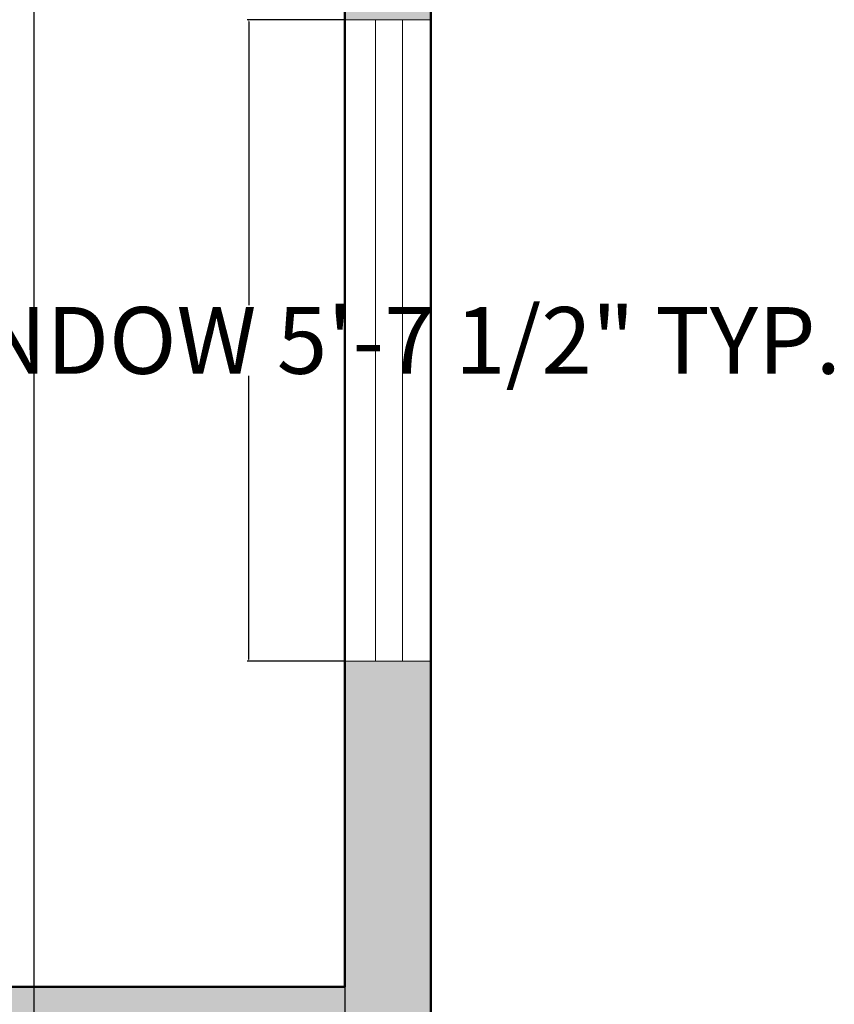
# Model space of a CAD drawing. Units: inches. Extents: x 2974 to 3443, y 2405 to 2963.
# Tile 9 of 13: x 3341 to 3427, y 2607 to 2711. Entities that reach past the tile are written whole.
import ezdxf

# ---------------------------------------------------------------- set-up
doc = ezdxf.new("R2010")
doc.units = ezdxf.units.IN
doc.header["$MEASUREMENT"] = 0
doc.layers.get('0').update_dxf_attribs({"color": 251})
for name, color, linetype, lineweight in [('A-ANNO-DIMS', 2, 'Continuous', 18), ('A-WALL-PATT', 252, 'Continuous', 13), ('walls', 250, 'Continuous', 50), ('windows', 159, 'Continuous', 20)]:
    doc.layers.add(name, color=color, linetype=linetype, lineweight=lineweight)
doc.styles.get("Standard").update_dxf_attribs({"font": 'arial.ttf'})
doc.dimstyles.get("Standard").update_dxf_attribs({"dimtxt": 7, "dimasz": 0.18, "dimexe": 0.18, "dimexo": 0.0625, "dimgap": 0.09, "dimtad": 0, "dimtih": 1, "dimtoh": 1, "dimzin": 0, "dimdsep": 46, "dimlunit": 3, "dimtxsty": 'Standard', "dimcen": 0.09, "dimadec": 0, "dimazin": 0, "dimtfac": 1, "dimtofl": 0, "dimtmove": 0, "dimatfit": 3, "dimfxl": 1, "dimtolj": 1, "dimtzin": 0, "dimarcsym": 0})

# ---------------------------------------------------------------- blocks, each defined once
blk = doc.blocks.new('WIN-67IN')
for p, q in [((0, 0), (9, 0)), ((0, -67.29), (0, 0)), ((0, 0), (3.19, 0)), ((3.19, 0), (3.19, -67.29)), ((6.02, -67.29), (6.02, 0)), ((9, 0), (9, -67.29)), ((9, -67.29), (0, -67.29)), ((3.19, -67.29), (6.02, -67.29))]:
    blk.add_line(p, q)
blk = doc.blocks.new('*D31')
at = {"layer": 'A-ANNO-DIMS', "color": 0, "lineweight": -2, "transparency": 16777216}
for p, q in [((3375.26, 2710.65), (3365.05, 2710.65)), ((3365.23, 2710.47), (3365.23, 2680.72)), ((3365.23, 2643.54), (3365.23, 2673.3)), ((3375.26, 2643.36), (3365.05, 2643.36))]:
    blk.add_line(p, q, dxfattribs=at)
at = {"layer": 'A-ANNO-DIMS', "color": 0, "transparency": 16777216}
for points in [[(3365.2, 2710.47), (3365.26, 2710.47), (3365.23, 2710.65)], [(3365.2, 2643.54), (3365.26, 2643.54), (3365.23, 2643.36)]]:
    blk.add_solid(points, dxfattribs=at)
at = {"layer": 'Defpoints', "color": 0, "transparency": 16777216}
for p in [(3365.23, 2710.65), (3375.33, 2710.65), (3375.33, 2643.36)]:
    blk.add_point(p, dxfattribs=at)
at = {"layer": 'A-ANNO-DIMS', "color": 0, "transparency": 16777216, "insert": (3365.23, 2677.01), "char_height": 7, "attachment_point": 5}
blk.add_mtext('\\A1;SIDE WINDOW 5\'-7 1/2" TYP.', dxfattribs=at)
blk = doc.blocks.new('*D32')
at = {"layer": 'A-ANNO-DIMS', "color": 0, "lineweight": -2, "transparency": 16777216}
for p, q in [((3375.33, 2710.72), (3375.33, 2720.93)), ((3375.51, 2720.75), (3384.15, 2720.75)), ((3384.33, 2710.72), (3384.33, 2720.93)), ((3384.33, 2720.75), (3384.51, 2720.75))]:
    blk.add_line(p, q, dxfattribs=at)
at = {"layer": 'A-ANNO-DIMS', "color": 0, "transparency": 16777216}
for points in [[(3375.51, 2720.78), (3375.51, 2720.72), (3375.33, 2720.75)], [(3384.15, 2720.78), (3384.15, 2720.72), (3384.33, 2720.75)]]:
    blk.add_solid(points, dxfattribs=at)
at = {"layer": 'Defpoints', "color": 0, "transparency": 16777216}
for p in [(3384.33, 2720.75), (3375.33, 2710.65), (3384.33, 2710.65)]:
    blk.add_point(p, dxfattribs=at)
at = {"layer": 'A-ANNO-DIMS', "color": 0, "transparency": 16777216, "insert": (3405.93, 2720.75), "char_height": 7, "attachment_point": 5}
blk.add_mtext('\\A1;0\'-9" TYP.', dxfattribs=at)
blk = doc.blocks.new('*D72')
at = {"layer": 'A-ANNO-DIMS', "color": 0, "lineweight": -2, "transparency": 16777216}
for p, q in [((3342.69, 2510.82), (3342.69, 2952.68)), ((3342.87, 2952.5), (3375.15, 2952.5)), ((3375.33, 2480.25), (3375.33, 2952.68)), ((3375.33, 2952.5), (3375.51, 2952.5))]:
    blk.add_line(p, q, dxfattribs=at)
at = {"layer": 'A-ANNO-DIMS', "color": 0, "transparency": 16777216}
for points in [[(3342.87, 2952.53), (3342.87, 2952.47), (3342.69, 2952.5)], [(3375.15, 2952.53), (3375.15, 2952.47), (3375.33, 2952.5)]]:
    blk.add_solid(points, dxfattribs=at)
at = {"layer": 'Defpoints', "color": 0, "transparency": 16777216}
for p in [(3375.33, 2952.5), (3342.69, 2510.76), (3375.33, 2480.19)]:
    blk.add_point(p, dxfattribs=at)
at = {"layer": 'A-ANNO-DIMS', "color": 0, "transparency": 16777216, "insert": (3393.11, 2952.5), "char_height": 7, "attachment_point": 5}
blk.add_mtext('\\A1;2\'-8 1/2"', dxfattribs=at)

msp = doc.modelspace()

# ---------------------------------------------------------------- hatches: boundary and pattern name
at = {"layer": 'A-WALL-PATT'}
h = msp.add_hatch(color=256, dxfattribs=at)
h.dxf.hatch_style = 1
h.paths.add_polyline_path([(3222.294, 2555.188), (3211.826, 2555.188), (3211.826, 2657.938), (3207.326, 2657.938), (3207.326, 2555.188), (3051.326, 2555.188), (3051.326, 2583.943), (3042.326, 2583.943), (3042.326, 2471.188), (3165.027, 2471.188), (3165.027, 2480.188), (3051.326, 2480.188), (3051.326, 2550.688), (3222.294, 2550.688)])
h.paths.add_polyline_path([(3188.326, 2700.207), (3183.826, 2700.207), (3183.826, 2691.688), (3051.326, 2691.688), (3051.326, 2740.572), (3042.326, 2740.572), (3042.326, 2651.235), (3045.517, 2651.235), (3051.326, 2651.235), (3051.326, 2687.188), (3188.326, 2687.188)])
h.paths.add_polyline_path([(3051.326, 2894.188), (3074.298, 2894.188), (3074.298, 2903.188), (3042.326, 2903.188), (3042.326, 2807.864), (3045.517, 2807.864), (3051.326, 2807.864), (3051.326, 2835.688), (3103.457, 2835.688), (3103.457, 2839.066, -0.0124729), (3103.485, 2840.188), (3051.326, 2840.188)])
h.paths.add_polyline_path([(3201.987, 2903.188), (3100.263, 2903.188), (3100.263, 2894.188), (3131.326, 2894.188), (3131.326, 2835.688), (3135.826, 2835.688), (3135.826, 2894.188), (3183.826, 2894.188), (3183.826, 2840.188), (3159.826, 2840.188), (3159.826, 2835.688), (3183.826, 2835.688), (3183.826, 2740.207), (3188.326, 2740.207), (3188.326, 2803.688), (3215.422, 2803.688), (3215.422, 2807.066, -0.0124729), (3215.45, 2808.188), (3188.326, 2808.188), (3188.326, 2894.188), (3201.987, 2894.188)])
h.paths.add_polyline_path([(3283.564, 2903.188), (3227.952, 2903.188), (3227.952, 2894.188), (3240.326, 2894.188), (3240.326, 2755.688), (3188.326, 2755.688), (3188.326, 2751.188), (3244.826, 2751.188), (3244.826, 2757.188), (3244.826, 2797.188), (3244.826, 2894.188), (3283.564, 2894.188)])
h.paths.add_polyline_path([(3384.326, 2903.188), (3346.694, 2903.188), (3346.694, 2894.188), (3375.326, 2894.188), (3375.326, 2755.688), (3284.826, 2755.688), (3284.826, 2751.188), (3375.326, 2751.188), (3375.326, 2710.653), (3378.517, 2710.653), (3384.326, 2710.653)])
h.paths.add_polyline_path([(3384.326, 2643.361), (3375.326, 2643.361), (3375.326, 2609.188), (3330.003, 2609.188), (3330.003, 2604.688), (3375.326, 2604.688), (3375.326, 2480.188), (3356.49, 2480.188), (3356.49, 2471.188), (3384.326, 2471.188)])
h.paths.add_polyline_path([(3267.326, 2609.188), (3262.826, 2609.188), (3262.826, 2555.188), (3257.429, 2555.188), (3257.429, 2550.688), (3262.826, 2550.688), (3262.826, 2471.188), (3293.36, 2471.188), (3293.36, 2480.188), (3267.326, 2480.188)])
h.paths.add_polyline_path([(3275.186, 2471.188), (3268.471, 2471.188), (3268.471, 2455.229), (3268.471, 2452.413), (3275.186, 2452.413)])
h.paths.add_polyline_path([(3156.684, 2471.188), (3149.969, 2471.188), (3149.969, 2452.413), (3156.684, 2452.413)])

# ---------------------------------------------------------------- linework, layer by layer
at = {"layer": 'walls'}
for p, q in [((3384.326, 2903.188), (3384.326, 2471.188)), ((3375.326, 2751.188), (3375.326, 2609.188)), ((3330.003, 2609.188), (3375.326, 2609.188))]:
    msp.add_line(p, q, dxfattribs=at)

# ---------------------------------------------------------------- block references
at = {"layer": 'windows'}
msp.add_blockref('WIN-67IN', (3375.326, 2710.653), dxfattribs=at)

# ---------------------------------------------------------------- dimensions: what is measured, and where the dimension line sits
at = {"layer": 'A-ANNO-DIMS'}
dim = msp.add_linear_dim(base=(3375.326, 2952.498), p1=(3342.691, 2510.762), p2=(3375.326, 2480.188), dimstyle='Standard', override={"dimdec": 1, "dimlfac": 1, "dimrnd": 0, "dimzin": 1, "dimdsep": 46, "dimlunit": 4, "dimfrac": 2}, dxfattribs=at)
dim.commit()
dim.dimension.update_dxf_attribs({"geometry": '*D72', "text_midpoint": (3393.115, 2952.498)})
dim = msp.add_linear_dim(base=(3384.326, 2720.747), p1=(3375.326, 2710.653), p2=(3384.326, 2710.653), text='<> TYP.', dimstyle='Standard', override={"dimdec": 1, "dimlfac": 1, "dimrnd": 0, "dimzin": 1, "dimdsep": 46, "dimlunit": 4, "dimfrac": 2}, dxfattribs=at)
dim.commit()
dim.dimension.update_dxf_attribs({"geometry": '*D32', "text_midpoint": (3405.93, 2720.747)})
dim = msp.add_linear_dim(base=(3365.232, 2710.653), p1=(3375.326, 2643.361), p2=(3375.326, 2710.653), angle=90, text='SIDE WINDOW <> TYP.', dimstyle='Standard', override={"dimdec": 1, "dimlfac": 1, "dimrnd": 0, "dimzin": 1, "dimdsep": 46, "dimlunit": 4, "dimfrac": 2}, dxfattribs=at)
dim.commit()
dim.dimension.update_dxf_attribs({"geometry": '*D31', "text_midpoint": (3365.232, 2677.007)})

doc.saveas('drawing.dxf')
